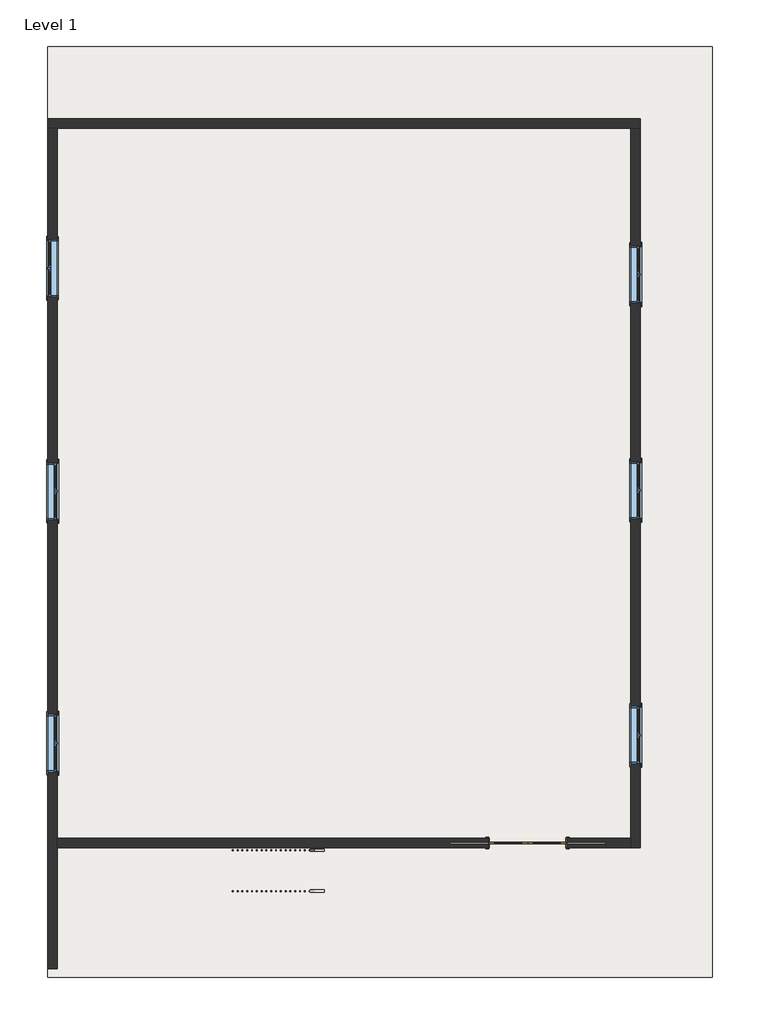
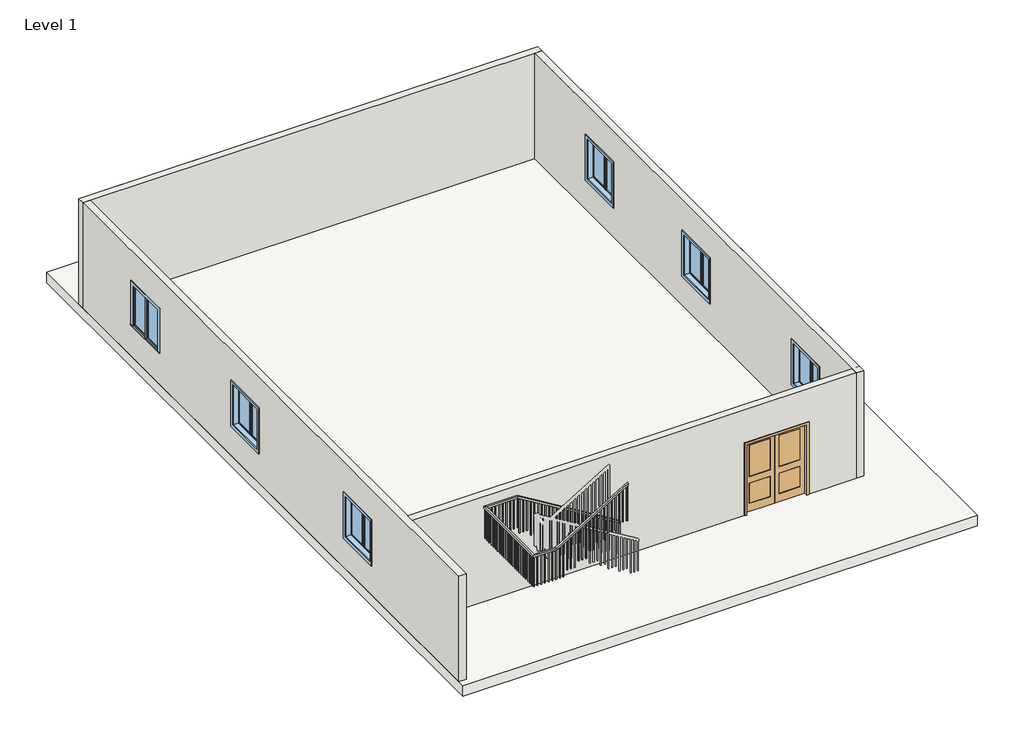
# One storey, part 1 of 2: 12 windows, 8 walls, 2 doors, 1 railing, 1 slab.
"""IFC4 building model written with IfcOpenShell, lengths in millimetres."""

from ifc_helpers import new_model, si_unit, frame, origin, origin_with_axes, place, context, project, spatial, polyline, outline, extrude, faceted_brep, transform, mapped, element, save
from components import door_18a53484, window_0862ab64

model = new_model("IFC4")

# Units and contexts
model_context = context("Model", 3, world=origin())
ifc_project = project(units=[si_unit("LENGTHUNIT", "METRE", prefix="MILLI")], contexts=[model_context])

# Site, building, storey
site = spatial("IfcSite", under=ifc_project)
building = spatial("IfcBuilding", under=site)
storey = spatial("IfcBuildingStorey", under=building, Name="Level 1", Elevation=0.0)

# Doors
placement = place(None, origin())
door_shape = door_18a53484(model_context)
element("IfcDoor", 1, ObjectType="Door-Interior-Double-Pocket-2_Panel-Wood : 64\" x 80\"", at=placement, inside=storey, context=model_context, shape_type="MappedRepresentation", body=[
    mapped(door_shape, transform((-1633.6127533, -5879.8242744, 0.0), x_axis=(1.0, 0.0, 0.0), y_axis=(0.0, 1.0, 0.0), z_axis=(0.0, 0.0, 1.0))),
])
element("IfcDoor", 2, ObjectType="Door-Interior-Double-Pocket-2_Panel-Wood : 64\" x 80\"", at=placement, inside=storey, context=model_context, shape_type="MappedRepresentation", body=[
    mapped(door_shape, transform((-1633.6127533, -5879.8242744, 0.0), x_axis=(1.0, 0.0, 0.0), y_axis=(0.0, 1.0, 0.0), z_axis=(0.0, 0.0, 1.0))),
])

# Railing
element("IfcRailing", 3, ObjectType="Handrail - Rectangular", at=placement, inside=storey, context=model_context, shape_type="SolidModel", body=[
    faceted_brep([(-5944.3382419, -6057.6242744, 1083.7333333), (-5944.3382419, -6057.6242744, 1024.3318731), (-5944.3382419, -6006.8242744, 1024.3318731), (-5944.3382419, -6006.8242744, 1083.7333333), (-8738.3382419, -6057.6242744, 2777.0666667), (-8752.5306513, -6057.6242744, 2726.2666667), (-8752.5306513, -6006.8242744, 2726.2666667), (-8738.3382419, -6006.8242744, 2777.0666667), (-9601.9382419, -6057.6242744, 2777.0666667), (-9601.9382419, -6057.6242744, 2726.2666667), (-9652.7382419, -6006.8242744, 2726.2666667), (-9652.7382419, -6006.8242744, 2777.0666667), (-9601.9382419, -8306.1243151, 2777.0666667), (-9601.9382419, -8306.1243151, 2726.2666667), (-9652.7382419, -8356.9243151, 2726.2666667), (-9652.7382419, -8356.9243151, 2777.0666667), (-9017.7382419, -8306.1243151, 2777.0666667), (-9003.5458325, -8306.1243151, 2726.2666667), (-9003.5458325, -8356.9243151, 2726.2666667), (-9017.7382419, -8356.9243151, 2777.0666667), (-7061.9382419, -8306.1243151, 3962.4), (-7061.9382419, -8356.9243151, 3962.4), (-7061.9382419, -8356.9243151, 3902.9985397), (-7061.9382419, -8306.1243151, 3902.9985397)], [[[0, 1, 2, 3]], [[1, 0, 4, 5]], [[2, 1, 5, 6]], [[3, 2, 6, 7]], [[0, 3, 7, 4]], [[5, 4, 8, 9]], [[6, 5, 9, 10]], [[7, 6, 10, 11]], [[4, 7, 11, 8]], [[9, 8, 12, 13]], [[10, 9, 13, 14]], [[11, 10, 14, 15]], [[8, 11, 15, 12]], [[13, 12, 16, 17]], [[14, 13, 17, 18]], [[15, 14, 18, 19]], [[12, 15, 19, 16]], [[20, 21, 22, 23]], [[17, 16, 20, 23]], [[18, 17, 23, 22]], [[19, 18, 22, 21]], [[16, 19, 21, 20]]]),
    extrude(outline(polyline([(3893.3773276, -7077.8132419), (3881.8318731, -7096.8632419), (2878.6666667, -7096.8632419), (2878.6666667, -7077.8132419), (3893.3773276, -7077.8132419)])), frame((0.0, -8341.0493151, 0.0), z_axis=(0.0, 1.0, 0.0), x_axis=(0.0, 0.0, 1.0)), (0.0, 0.0, 1.0), 19.05),
    extrude(outline(polyline([(3831.80157, -7179.4132419), (3820.2561155, -7198.4632419), (2878.6666667, -7198.4632419), (2878.6666667, -7179.4132419), (3831.80157, -7179.4132419)])), frame((0.0, -8341.0493151, 0.0), z_axis=(0.0, 1.0, 0.0), x_axis=(0.0, 0.0, 1.0)), (0.0, 0.0, 1.0), 19.05),
    extrude(outline(polyline([(3770.2258125, -7281.0132419), (3758.6803579, -7300.0632419), (2878.6666667, -7300.0632419), (2878.6666667, -7281.0132419), (3770.2258125, -7281.0132419)])), frame((0.0, -8341.0493151, 0.0), z_axis=(0.0, 1.0, 0.0), x_axis=(0.0, 0.0, 1.0)), (0.0, 0.0, 1.0), 19.05),
    extrude(outline(polyline([(3708.6500549, -7382.6132419), (3697.1046004, -7401.6632419), (2709.3333333, -7401.6632419), (2709.3333333, -7382.6132419), (3708.6500549, -7382.6132419)])), frame((0.0, -8341.0493151, 0.0), z_axis=(0.0, 1.0, 0.0), x_axis=(0.0, 0.0, 1.0)), (0.0, 0.0, 1.0), 19.05),
    extrude(outline(polyline([(3647.0742973, -7484.2132419), (3635.5288428, -7503.2632419), (2709.3333333, -7503.2632419), (2709.3333333, -7484.2132419), (3647.0742973, -7484.2132419)])), frame((0.0, -8341.0493151, 0.0), z_axis=(0.0, 1.0, 0.0), x_axis=(0.0, 0.0, 1.0)), (0.0, 0.0, 1.0), 19.05),
    extrude(outline(polyline([(3585.4985397, -7585.8132419), (3573.9530852, -7604.8632419), (2709.3333333, -7604.8632419), (2709.3333333, -7585.8132419), (3585.4985397, -7585.8132419)])), frame((0.0, -8341.0493151, 0.0), z_axis=(0.0, 1.0, 0.0), x_axis=(0.0, 0.0, 1.0)), (0.0, 0.0, 1.0), 19.05),
    extrude(outline(polyline([(3523.9227822, -7687.4132419), (3512.3773276, -7706.4632419), (2540.0, -7706.4632419), (2540.0, -7687.4132419), (3523.9227822, -7687.4132419)])), frame((0.0, -8341.0493151, 0.0), z_axis=(0.0, 1.0, 0.0), x_axis=(0.0, 0.0, 1.0)), (0.0, 0.0, 1.0), 19.05),
    extrude(outline(polyline([(3462.3470246, -7789.0132419), (3450.80157, -7808.0632419), (2540.0, -7808.0632419), (2540.0, -7789.0132419), (3462.3470246, -7789.0132419)])), frame((0.0, -8341.0493151, 0.0), z_axis=(0.0, 1.0, 0.0), x_axis=(0.0, 0.0, 1.0)), (0.0, 0.0, 1.0), 19.05),
    extrude(outline(polyline([(3400.771267, -7890.6132419), (3389.2258125, -7909.6632419), (2540.0, -7909.6632419), (2540.0, -7890.6132419), (3400.771267, -7890.6132419)])), frame((0.0, -8341.0493151, 0.0), z_axis=(0.0, 1.0, 0.0), x_axis=(0.0, 0.0, 1.0)), (0.0, 0.0, 1.0), 19.05),
    extrude(outline(polyline([(3339.1955094, -7992.2132419), (3327.6500549, -8011.2632419), (2370.6666667, -8011.2632419), (2370.6666667, -7992.2132419), (3339.1955094, -7992.2132419)])), frame((0.0, -8341.0493151, 0.0), z_axis=(0.0, 1.0, 0.0), x_axis=(0.0, 0.0, 1.0)), (0.0, 0.0, 1.0), 19.05),
    extrude(outline(polyline([(3277.6197519, -8093.8132419), (3266.0742973, -8112.8632419), (2370.6666667, -8112.8632419), (2370.6666667, -8093.8132419), (3277.6197519, -8093.8132419)])), frame((0.0, -8341.0493151, 0.0), z_axis=(0.0, 1.0, 0.0), x_axis=(0.0, 0.0, 1.0)), (0.0, 0.0, 1.0), 19.05),
    extrude(outline(polyline([(3216.0439943, -8195.4132419), (3204.4985397, -8214.4632419), (2201.3333333, -8214.4632419), (2201.3333333, -8195.4132419), (3216.0439943, -8195.4132419)])), frame((0.0, -8341.0493151, 0.0), z_axis=(0.0, 1.0, 0.0), x_axis=(0.0, 0.0, 1.0)), (0.0, 0.0, 1.0), 19.05),
    extrude(outline(polyline([(3154.4682367, -8297.0132419), (3142.9227822, -8316.0632419), (2201.3333333, -8316.0632419), (2201.3333333, -8297.0132419), (3154.4682367, -8297.0132419)])), frame((0.0, -8341.0493151, 0.0), z_axis=(0.0, 1.0, 0.0), x_axis=(0.0, 0.0, 1.0)), (0.0, 0.0, 1.0), 19.05),
    extrude(outline(polyline([(3092.8924791, -8398.6132419), (3081.3470246, -8417.6632419), (2201.3333333, -8417.6632419), (2201.3333333, -8398.6132419), (3092.8924791, -8398.6132419)])), frame((0.0, -8341.0493151, 0.0), z_axis=(0.0, 1.0, 0.0), x_axis=(0.0, 0.0, 1.0)), (0.0, 0.0, 1.0), 19.05),
    extrude(outline(polyline([(3031.3167216, -8500.2132419), (3019.771267, -8519.2632419), (2032.0, -8519.2632419), (2032.0, -8500.2132419), (3031.3167216, -8500.2132419)])), frame((0.0, -8341.0493151, 0.0), z_axis=(0.0, 1.0, 0.0), x_axis=(0.0, 0.0, 1.0)), (0.0, 0.0, 1.0), 19.05),
    extrude(outline(polyline([(2969.740964, -8601.8132419), (2958.1955094, -8620.8632419), (2032.0, -8620.8632419), (2032.0, -8601.8132419), (2969.740964, -8601.8132419)])), frame((0.0, -8341.0493151, 0.0), z_axis=(0.0, 1.0, 0.0), x_axis=(0.0, 0.0, 1.0)), (0.0, 0.0, 1.0), 19.05),
    extrude(outline(polyline([(2908.1652064, -8703.4132419), (2896.6197519, -8722.4632419), (2032.0, -8722.4632419), (2032.0, -8703.4132419), (2908.1652064, -8703.4132419)])), frame((0.0, -8341.0493151, 0.0), z_axis=(0.0, 1.0, 0.0), x_axis=(0.0, 0.0, 1.0)), (0.0, 0.0, 1.0), 19.05),
    extrude(outline(polyline([(2846.5894488, -8805.0132419), (2835.0439943, -8824.0632419), (1862.6666667, -8824.0632419), (1862.6666667, -8805.0132419), (2846.5894488, -8805.0132419)])), frame((0.0, -8341.0493151, 0.0), z_axis=(0.0, 1.0, 0.0), x_axis=(0.0, 0.0, 1.0)), (0.0, 0.0, 1.0), 19.05),
    extrude(outline(polyline([(2785.0136913, -8906.6132419), (2773.4682367, -8925.6632419), (1862.6666667, -8925.6632419), (1862.6666667, -8906.6132419), (2785.0136913, -8906.6132419)])), frame((0.0, -8341.0493151, 0.0), z_axis=(0.0, 1.0, 0.0), x_axis=(0.0, 0.0, 1.0)), (0.0, 0.0, 1.0), 19.05),
    extrude(outline(polyline([(-9128.8632419, -8341.0493151), (-9128.8632419, -8321.9993151), (-9109.8132419, -8321.9993151), (-9109.8132419, -8341.0493151), (-9128.8632419, -8341.0493151)])), frame((0.0, 0.0, 1862.6666667), z_axis=(0.0, 0.0, 1.0), x_axis=(1.0, 0.0, 0.0)), (0.0, 0.0, 1.0), 863.6),
    extrude(outline(polyline([(-9230.4632419, -8341.0493151), (-9230.4632419, -8321.9993151), (-9211.4132419, -8321.9993151), (-9211.4132419, -8341.0493151), (-9230.4632419, -8341.0493151)])), frame((0.0, 0.0, 1862.6666667), z_axis=(0.0, 0.0, 1.0), x_axis=(1.0, 0.0, 0.0)), (0.0, 0.0, 1.0), 863.6),
    extrude(outline(polyline([(-9332.0632419, -8341.0493151), (-9332.0632419, -8321.9993151), (-9313.0132419, -8321.9993151), (-9313.0132419, -8341.0493151), (-9332.0632419, -8341.0493151)])), frame((0.0, 0.0, 1862.6666667), z_axis=(0.0, 0.0, 1.0), x_axis=(1.0, 0.0, 0.0)), (0.0, 0.0, 1.0), 863.6),
    extrude(outline(polyline([(-9433.6632419, -8341.0493151), (-9433.6632419, -8321.9993151), (-9414.6132419, -8321.9993151), (-9414.6132419, -8341.0493151), (-9433.6632419, -8341.0493151)])), frame((0.0, 0.0, 1862.6666667), z_axis=(0.0, 0.0, 1.0), x_axis=(1.0, 0.0, 0.0)), (0.0, 0.0, 1.0), 863.6),
    extrude(outline(polyline([(-9535.2632419, -8341.0493151), (-9535.2632419, -8321.9993151), (-9516.2132419, -8321.9993151), (-9516.2132419, -8341.0493151), (-9535.2632419, -8341.0493151)])), frame((0.0, 0.0, 1862.6666667), z_axis=(0.0, 0.0, 1.0), x_axis=(1.0, 0.0, 0.0)), (0.0, 0.0, 1.0), 863.6),
    extrude(outline(polyline([(-9636.8632419, -8257.8992744), (-9617.8132419, -8257.8992744), (-9617.8132419, -8276.9492744), (-9636.8632419, -8276.9492744), (-9636.8632419, -8257.8992744)])), frame((0.0, 0.0, 1862.6666667), z_axis=(0.0, 0.0, 1.0), x_axis=(1.0, 0.0, 0.0)), (0.0, 0.0, 1.0), 863.6),
    extrude(outline(polyline([(-9636.8632419, -8156.2992744), (-9617.8132419, -8156.2992744), (-9617.8132419, -8175.3492744), (-9636.8632419, -8175.3492744), (-9636.8632419, -8156.2992744)])), frame((0.0, 0.0, 1862.6666667), z_axis=(0.0, 0.0, 1.0), x_axis=(1.0, 0.0, 0.0)), (0.0, 0.0, 1.0), 863.6),
    extrude(outline(polyline([(-9636.8632419, -8054.6992744), (-9617.8132419, -8054.6992744), (-9617.8132419, -8073.7492744), (-9636.8632419, -8073.7492744), (-9636.8632419, -8054.6992744)])), frame((0.0, 0.0, 1862.6666667), z_axis=(0.0, 0.0, 1.0), x_axis=(1.0, 0.0, 0.0)), (0.0, 0.0, 1.0), 863.6),
    extrude(outline(polyline([(-9636.8632419, -7953.0992744), (-9617.8132419, -7953.0992744), (-9617.8132419, -7972.1492744), (-9636.8632419, -7972.1492744), (-9636.8632419, -7953.0992744)])), frame((0.0, 0.0, 1862.6666667), z_axis=(0.0, 0.0, 1.0), x_axis=(1.0, 0.0, 0.0)), (0.0, 0.0, 1.0), 863.6),
    extrude(outline(polyline([(-9636.8632419, -7851.4992744), (-9617.8132419, -7851.4992744), (-9617.8132419, -7870.5492744), (-9636.8632419, -7870.5492744), (-9636.8632419, -7851.4992744)])), frame((0.0, 0.0, 1862.6666667), z_axis=(0.0, 0.0, 1.0), x_axis=(1.0, 0.0, 0.0)), (0.0, 0.0, 1.0), 863.6),
    extrude(outline(polyline([(-9636.8632419, -7749.8992744), (-9617.8132419, -7749.8992744), (-9617.8132419, -7768.9492744), (-9636.8632419, -7768.9492744), (-9636.8632419, -7749.8992744)])), frame((0.0, 0.0, 1862.6666667), z_axis=(0.0, 0.0, 1.0), x_axis=(1.0, 0.0, 0.0)), (0.0, 0.0, 1.0), 863.6),
    extrude(outline(polyline([(-9636.8632419, -7648.2992744), (-9617.8132419, -7648.2992744), (-9617.8132419, -7667.3492744), (-9636.8632419, -7667.3492744), (-9636.8632419, -7648.2992744)])), frame((0.0, 0.0, 1862.6666667), z_axis=(0.0, 0.0, 1.0), x_axis=(1.0, 0.0, 0.0)), (0.0, 0.0, 1.0), 863.6),
    extrude(outline(polyline([(-9636.8632419, -7546.6992744), (-9617.8132419, -7546.6992744), (-9617.8132419, -7565.7492744), (-9636.8632419, -7565.7492744), (-9636.8632419, -7546.6992744)])), frame((0.0, 0.0, 1862.6666667), z_axis=(0.0, 0.0, 1.0), x_axis=(1.0, 0.0, 0.0)), (0.0, 0.0, 1.0), 863.6),
    extrude(outline(polyline([(-9636.8632419, -7445.0992744), (-9617.8132419, -7445.0992744), (-9617.8132419, -7464.1492744), (-9636.8632419, -7464.1492744), (-9636.8632419, -7445.0992744)])), frame((0.0, 0.0, 1862.6666667), z_axis=(0.0, 0.0, 1.0), x_axis=(1.0, 0.0, 0.0)), (0.0, 0.0, 1.0), 863.6),
    extrude(outline(polyline([(-9636.8632419, -7343.4992744), (-9617.8132419, -7343.4992744), (-9617.8132419, -7362.5492744), (-9636.8632419, -7362.5492744), (-9636.8632419, -7343.4992744)])), frame((0.0, 0.0, 1862.6666667), z_axis=(0.0, 0.0, 1.0), x_axis=(1.0, 0.0, 0.0)), (0.0, 0.0, 1.0), 863.6),
    extrude(outline(polyline([(-9636.8632419, -7241.8992744), (-9617.8132419, -7241.8992744), (-9617.8132419, -7260.9492744), (-9636.8632419, -7260.9492744), (-9636.8632419, -7241.8992744)])), frame((0.0, 0.0, 1862.6666667), z_axis=(0.0, 0.0, 1.0), x_axis=(1.0, 0.0, 0.0)), (0.0, 0.0, 1.0), 863.6),
    extrude(outline(polyline([(-9636.8632419, -7140.2992744), (-9617.8132419, -7140.2992744), (-9617.8132419, -7159.3492744), (-9636.8632419, -7159.3492744), (-9636.8632419, -7140.2992744)])), frame((0.0, 0.0, 1862.6666667), z_axis=(0.0, 0.0, 1.0), x_axis=(1.0, 0.0, 0.0)), (0.0, 0.0, 1.0), 863.6),
    extrude(outline(polyline([(-9636.8632419, -7038.6992744), (-9617.8132419, -7038.6992744), (-9617.8132419, -7057.7492744), (-9636.8632419, -7057.7492744), (-9636.8632419, -7038.6992744)])), frame((0.0, 0.0, 1862.6666667), z_axis=(0.0, 0.0, 1.0), x_axis=(1.0, 0.0, 0.0)), (0.0, 0.0, 1.0), 863.6),
    extrude(outline(polyline([(-9636.8632419, -6937.0992744), (-9617.8132419, -6937.0992744), (-9617.8132419, -6956.1492744), (-9636.8632419, -6956.1492744), (-9636.8632419, -6937.0992744)])), frame((0.0, 0.0, 1862.6666667), z_axis=(0.0, 0.0, 1.0), x_axis=(1.0, 0.0, 0.0)), (0.0, 0.0, 1.0), 863.6),
    extrude(outline(polyline([(-9636.8632419, -6835.4992744), (-9617.8132419, -6835.4992744), (-9617.8132419, -6854.5492744), (-9636.8632419, -6854.5492744), (-9636.8632419, -6835.4992744)])), frame((0.0, 0.0, 1862.6666667), z_axis=(0.0, 0.0, 1.0), x_axis=(1.0, 0.0, 0.0)), (0.0, 0.0, 1.0), 863.6),
    extrude(outline(polyline([(-9636.8632419, -6733.8992744), (-9617.8132419, -6733.8992744), (-9617.8132419, -6752.9492744), (-9636.8632419, -6752.9492744), (-9636.8632419, -6733.8992744)])), frame((0.0, 0.0, 1862.6666667), z_axis=(0.0, 0.0, 1.0), x_axis=(1.0, 0.0, 0.0)), (0.0, 0.0, 1.0), 863.6),
    extrude(outline(polyline([(-9636.8632419, -6632.2992744), (-9617.8132419, -6632.2992744), (-9617.8132419, -6651.3492744), (-9636.8632419, -6651.3492744), (-9636.8632419, -6632.2992744)])), frame((0.0, 0.0, 1862.6666667), z_axis=(0.0, 0.0, 1.0), x_axis=(1.0, 0.0, 0.0)), (0.0, 0.0, 1.0), 863.6),
    extrude(outline(polyline([(-9636.8632419, -6530.6992744), (-9617.8132419, -6530.6992744), (-9617.8132419, -6549.7492744), (-9636.8632419, -6549.7492744), (-9636.8632419, -6530.6992744)])), frame((0.0, 0.0, 1862.6666667), z_axis=(0.0, 0.0, 1.0), x_axis=(1.0, 0.0, 0.0)), (0.0, 0.0, 1.0), 863.6),
    extrude(outline(polyline([(-9636.8632419, -6429.0992744), (-9617.8132419, -6429.0992744), (-9617.8132419, -6448.1492744), (-9636.8632419, -6448.1492744), (-9636.8632419, -6429.0992744)])), frame((0.0, 0.0, 1862.6666667), z_axis=(0.0, 0.0, 1.0), x_axis=(1.0, 0.0, 0.0)), (0.0, 0.0, 1.0), 863.6),
    extrude(outline(polyline([(-9636.8632419, -6327.4992744), (-9617.8132419, -6327.4992744), (-9617.8132419, -6346.5492744), (-9636.8632419, -6346.5492744), (-9636.8632419, -6327.4992744)])), frame((0.0, 0.0, 1862.6666667), z_axis=(0.0, 0.0, 1.0), x_axis=(1.0, 0.0, 0.0)), (0.0, 0.0, 1.0), 863.6),
    extrude(outline(polyline([(-9636.8632419, -6225.8992744), (-9617.8132419, -6225.8992744), (-9617.8132419, -6244.9492744), (-9636.8632419, -6244.9492744), (-9636.8632419, -6225.8992744)])), frame((0.0, 0.0, 1862.6666667), z_axis=(0.0, 0.0, 1.0), x_axis=(1.0, 0.0, 0.0)), (0.0, 0.0, 1.0), 863.6),
    extrude(outline(polyline([(-9636.8632419, -6124.2992744), (-9617.8132419, -6124.2992744), (-9617.8132419, -6143.3492744), (-9636.8632419, -6143.3492744), (-9636.8632419, -6124.2992744)])), frame((0.0, 0.0, 1862.6666667), z_axis=(0.0, 0.0, 1.0), x_axis=(1.0, 0.0, 0.0)), (0.0, 0.0, 1.0), 863.6),
    extrude(outline(polyline([(-9541.6132419, -6022.6992744), (-9541.6132419, -6041.7492744), (-9560.6632419, -6041.7492744), (-9560.6632419, -6022.6992744), (-9541.6132419, -6022.6992744)])), frame((0.0, 0.0, 1862.6666667), z_axis=(0.0, 0.0, 1.0), x_axis=(1.0, 0.0, 0.0)), (0.0, 0.0, 1.0), 863.6),
    extrude(outline(polyline([(-9440.0132419, -6022.6992744), (-9440.0132419, -6041.7492744), (-9459.0632419, -6041.7492744), (-9459.0632419, -6022.6992744), (-9440.0132419, -6022.6992744)])), frame((0.0, 0.0, 1862.6666667), z_axis=(0.0, 0.0, 1.0), x_axis=(1.0, 0.0, 0.0)), (0.0, 0.0, 1.0), 863.6),
    extrude(outline(polyline([(-9338.4132419, -6022.6992744), (-9338.4132419, -6041.7492744), (-9357.4632419, -6041.7492744), (-9357.4632419, -6022.6992744), (-9338.4132419, -6022.6992744)])), frame((0.0, 0.0, 1862.6666667), z_axis=(0.0, 0.0, 1.0), x_axis=(1.0, 0.0, 0.0)), (0.0, 0.0, 1.0), 863.6),
    extrude(outline(polyline([(-9236.8132419, -6022.6992744), (-9236.8132419, -6041.7492744), (-9255.8632419, -6041.7492744), (-9255.8632419, -6022.6992744), (-9236.8132419, -6022.6992744)])), frame((0.0, 0.0, 1862.6666667), z_axis=(0.0, 0.0, 1.0), x_axis=(1.0, 0.0, 0.0)), (0.0, 0.0, 1.0), 863.6),
    extrude(outline(polyline([(-9135.2132419, -6022.6992744), (-9135.2132419, -6041.7492744), (-9154.2632419, -6041.7492744), (-9154.2632419, -6022.6992744), (-9135.2132419, -6022.6992744)])), frame((0.0, 0.0, 1862.6666667), z_axis=(0.0, 0.0, 1.0), x_axis=(1.0, 0.0, 0.0)), (0.0, 0.0, 1.0), 863.6),
    extrude(outline(polyline([(-9033.6132419, -6022.6992744), (-9033.6132419, -6041.7492744), (-9052.6632419, -6041.7492744), (-9052.6632419, -6022.6992744), (-9033.6132419, -6022.6992744)])), frame((0.0, 0.0, 1862.6666667), z_axis=(0.0, 0.0, 1.0), x_axis=(1.0, 0.0, 0.0)), (0.0, 0.0, 1.0), 863.6),
    extrude(outline(polyline([(-8932.0132419, -6022.6992744), (-8932.0132419, -6041.7492744), (-8951.0632419, -6041.7492744), (-8951.0632419, -6022.6992744), (-8932.0132419, -6022.6992744)])), frame((0.0, 0.0, 1862.6666667), z_axis=(0.0, 0.0, 1.0), x_axis=(1.0, 0.0, 0.0)), (0.0, 0.0, 1.0), 863.6),
    extrude(outline(polyline([(-8830.4132419, -6022.6992744), (-8830.4132419, -6041.7492744), (-8849.4632419, -6041.7492744), (-8849.4632419, -6022.6992744), (-8830.4132419, -6022.6992744)])), frame((0.0, 0.0, 1862.6666667), z_axis=(0.0, 0.0, 1.0), x_axis=(1.0, 0.0, 0.0)), (0.0, 0.0, 1.0), 863.6),
    extrude(outline(polyline([(2681.1046004, -8678.0132419), (2692.6500549, -8697.0632419), (1693.3333333, -8697.0632419), (1693.3333333, -8678.0132419), (2681.1046004, -8678.0132419)])), frame((0.0, -6041.7492744, 0.0), z_axis=(0.0, 1.0, 0.0), x_axis=(0.0, 0.0, 1.0)), (0.0, 0.0, 1.0), 19.05),
    extrude(outline(polyline([(2619.5288428, -8576.4132419), (2631.0742973, -8595.4632419), (1693.3333333, -8595.4632419), (1693.3333333, -8576.4132419), (2619.5288428, -8576.4132419)])), frame((0.0, -6041.7492744, 0.0), z_axis=(0.0, 1.0, 0.0), x_axis=(0.0, 0.0, 1.0)), (0.0, 0.0, 1.0), 19.05),
    extrude(outline(polyline([(2557.9530852, -8474.8132419), (2569.4985397, -8493.8632419), (1693.3333333, -8493.8632419), (1693.3333333, -8474.8132419), (2557.9530852, -8474.8132419)])), frame((0.0, -6041.7492744, 0.0), z_axis=(0.0, 1.0, 0.0), x_axis=(0.0, 0.0, 1.0)), (0.0, 0.0, 1.0), 19.05),
    extrude(outline(polyline([(2496.3773276, -8373.2132419), (2507.9227822, -8392.2632419), (1524.0, -8392.2632419), (1524.0, -8373.2132419), (2496.3773276, -8373.2132419)])), frame((0.0, -6041.7492744, 0.0), z_axis=(0.0, 1.0, 0.0), x_axis=(0.0, 0.0, 1.0)), (0.0, 0.0, 1.0), 19.05),
    extrude(outline(polyline([(2434.80157, -8271.6132419), (2446.3470246, -8290.6632419), (1524.0, -8290.6632419), (1524.0, -8271.6132419), (2434.80157, -8271.6132419)])), frame((0.0, -6041.7492744, 0.0), z_axis=(0.0, 1.0, 0.0), x_axis=(0.0, 0.0, 1.0)), (0.0, 0.0, 1.0), 19.05),
    extrude(outline(polyline([(2373.2258125, -8170.0132419), (2384.771267, -8189.0632419), (1524.0, -8189.0632419), (1524.0, -8170.0132419), (2373.2258125, -8170.0132419)])), frame((0.0, -6041.7492744, 0.0), z_axis=(0.0, 1.0, 0.0), x_axis=(0.0, 0.0, 1.0)), (0.0, 0.0, 1.0), 19.05),
    extrude(outline(polyline([(2311.6500549, -8068.4132419), (2323.1955094, -8087.4632419), (1354.6666667, -8087.4632419), (1354.6666667, -8068.4132419), (2311.6500549, -8068.4132419)])), frame((0.0, -6041.7492744, 0.0), z_axis=(0.0, 1.0, 0.0), x_axis=(0.0, 0.0, 1.0)), (0.0, 0.0, 1.0), 19.05),
    extrude(outline(polyline([(2250.0742973, -7966.8132419), (2261.6197519, -7985.8632419), (1354.6666667, -7985.8632419), (1354.6666667, -7966.8132419), (2250.0742973, -7966.8132419)])), frame((0.0, -6041.7492744, 0.0), z_axis=(0.0, 1.0, 0.0), x_axis=(0.0, 0.0, 1.0)), (0.0, 0.0, 1.0), 19.05),
    extrude(outline(polyline([(2188.4985397, -7865.2132419), (2200.0439943, -7884.2632419), (1185.3333333, -7884.2632419), (1185.3333333, -7865.2132419), (2188.4985397, -7865.2132419)])), frame((0.0, -6041.7492744, 0.0), z_axis=(0.0, 1.0, 0.0), x_axis=(0.0, 0.0, 1.0)), (0.0, 0.0, 1.0), 19.05),
    extrude(outline(polyline([(2126.9227822, -7763.6132419), (2138.4682367, -7782.6632419), (1185.3333333, -7782.6632419), (1185.3333333, -7763.6132419), (2126.9227822, -7763.6132419)])), frame((0.0, -6041.7492744, 0.0), z_axis=(0.0, 1.0, 0.0), x_axis=(0.0, 0.0, 1.0)), (0.0, 0.0, 1.0), 19.05),
    extrude(outline(polyline([(2065.3470246, -7662.0132419), (2076.8924791, -7681.0632419), (1185.3333333, -7681.0632419), (1185.3333333, -7662.0132419), (2065.3470246, -7662.0132419)])), frame((0.0, -6041.7492744, 0.0), z_axis=(0.0, 1.0, 0.0), x_axis=(0.0, 0.0, 1.0)), (0.0, 0.0, 1.0), 19.05),
    extrude(outline(polyline([(2003.771267, -7560.4132419), (2015.3167216, -7579.4632419), (1016.0, -7579.4632419), (1016.0, -7560.4132419), (2003.771267, -7560.4132419)])), frame((0.0, -6041.7492744, 0.0), z_axis=(0.0, 1.0, 0.0), x_axis=(0.0, 0.0, 1.0)), (0.0, 0.0, 1.0), 19.05),
    extrude(outline(polyline([(1942.1955094, -7458.8132419), (1953.740964, -7477.8632419), (1016.0, -7477.8632419), (1016.0, -7458.8132419), (1942.1955094, -7458.8132419)])), frame((0.0, -6041.7492744, 0.0), z_axis=(0.0, 1.0, 0.0), x_axis=(0.0, 0.0, 1.0)), (0.0, 0.0, 1.0), 19.05),
    extrude(outline(polyline([(1880.6197519, -7357.2132419), (1892.1652064, -7376.2632419), (1016.0, -7376.2632419), (1016.0, -7357.2132419), (1880.6197519, -7357.2132419)])), frame((0.0, -6041.7492744, 0.0), z_axis=(0.0, 1.0, 0.0), x_axis=(0.0, 0.0, 1.0)), (0.0, 0.0, 1.0), 19.05),
    extrude(outline(polyline([(1819.0439943, -7255.6132419), (1830.5894488, -7274.6632419), (846.6666667, -7274.6632419), (846.6666667, -7255.6132419), (1819.0439943, -7255.6132419)])), frame((0.0, -6041.7492744, 0.0), z_axis=(0.0, 1.0, 0.0), x_axis=(0.0, 0.0, 1.0)), (0.0, 0.0, 1.0), 19.05),
    extrude(outline(polyline([(1757.4682367, -7154.0132419), (1769.0136913, -7173.0632419), (846.6666667, -7173.0632419), (846.6666667, -7154.0132419), (1757.4682367, -7154.0132419)])), frame((0.0, -6041.7492744, 0.0), z_axis=(0.0, 1.0, 0.0), x_axis=(0.0, 0.0, 1.0)), (0.0, 0.0, 1.0), 19.05),
    extrude(outline(polyline([(1695.8924791, -7052.4132419), (1707.4379337, -7071.4632419), (846.6666667, -7071.4632419), (846.6666667, -7052.4132419), (1695.8924791, -7052.4132419)])), frame((0.0, -6041.7492744, 0.0), z_axis=(0.0, 1.0, 0.0), x_axis=(0.0, 0.0, 1.0)), (0.0, 0.0, 1.0), 19.05),
    extrude(outline(polyline([(1634.3167216, -6950.8132419), (1645.8621761, -6969.8632419), (677.3333333, -6969.8632419), (677.3333333, -6950.8132419), (1634.3167216, -6950.8132419)])), frame((0.0, -6041.7492744, 0.0), z_axis=(0.0, 1.0, 0.0), x_axis=(0.0, 0.0, 1.0)), (0.0, 0.0, 1.0), 19.05),
    extrude(outline(polyline([(1572.740964, -6849.2132419), (1584.2864185, -6868.2632419), (677.3333333, -6868.2632419), (677.3333333, -6849.2132419), (1572.740964, -6849.2132419)])), frame((0.0, -6041.7492744, 0.0), z_axis=(0.0, 1.0, 0.0), x_axis=(0.0, 0.0, 1.0)), (0.0, 0.0, 1.0), 19.05),
    extrude(outline(polyline([(1511.1652064, -6747.6132419), (1522.710661, -6766.6632419), (508.0, -6766.6632419), (508.0, -6747.6132419), (1511.1652064, -6747.6132419)])), frame((0.0, -6041.7492744, 0.0), z_axis=(0.0, 1.0, 0.0), x_axis=(0.0, 0.0, 1.0)), (0.0, 0.0, 1.0), 19.05),
    extrude(outline(polyline([(1449.5894488, -6646.0132419), (1461.1349034, -6665.0632419), (508.0, -6665.0632419), (508.0, -6646.0132419), (1449.5894488, -6646.0132419)])), frame((0.0, -6041.7492744, 0.0), z_axis=(0.0, 1.0, 0.0), x_axis=(0.0, 0.0, 1.0)), (0.0, 0.0, 1.0), 19.05),
    extrude(outline(polyline([(1388.0136913, -6544.4132419), (1399.5591458, -6563.4632419), (508.0, -6563.4632419), (508.0, -6544.4132419), (1388.0136913, -6544.4132419)])), frame((0.0, -6041.7492744, 0.0), z_axis=(0.0, 1.0, 0.0), x_axis=(0.0, 0.0, 1.0)), (0.0, 0.0, 1.0), 19.05),
    extrude(outline(polyline([(1326.4379337, -6442.8132419), (1337.9833882, -6461.8632419), (338.6666667, -6461.8632419), (338.6666667, -6442.8132419), (1326.4379337, -6442.8132419)])), frame((0.0, -6041.7492744, 0.0), z_axis=(0.0, 1.0, 0.0), x_axis=(0.0, 0.0, 1.0)), (0.0, 0.0, 1.0), 19.05),
    extrude(outline(polyline([(1264.8621761, -6341.2132419), (1276.4076307, -6360.2632419), (338.6666667, -6360.2632419), (338.6666667, -6341.2132419), (1264.8621761, -6341.2132419)])), frame((0.0, -6041.7492744, 0.0), z_axis=(0.0, 1.0, 0.0), x_axis=(0.0, 0.0, 1.0)), (0.0, 0.0, 1.0), 19.05),
    extrude(outline(polyline([(1203.2864185, -6239.6132419), (1214.8318731, -6258.6632419), (338.6666667, -6258.6632419), (338.6666667, -6239.6132419), (1203.2864185, -6239.6132419)])), frame((0.0, -6041.7492744, 0.0), z_axis=(0.0, 1.0, 0.0), x_axis=(0.0, 0.0, 1.0)), (0.0, 0.0, 1.0), 19.05),
    extrude(outline(polyline([(1141.710661, -6138.0132419), (1153.2561155, -6157.0632419), (169.3333333, -6157.0632419), (169.3333333, -6138.0132419), (1141.710661, -6138.0132419)])), frame((0.0, -6041.7492744, 0.0), z_axis=(0.0, 1.0, 0.0), x_axis=(0.0, 0.0, 1.0)), (0.0, 0.0, 1.0), 19.05),
    extrude(outline(polyline([(1080.1349034, -6036.4132419), (1091.6803579, -6055.4632419), (169.3333333, -6055.4632419), (169.3333333, -6036.4132419), (1080.1349034, -6036.4132419)])), frame((0.0, -6041.7492744, 0.0), z_axis=(0.0, 1.0, 0.0), x_axis=(0.0, 0.0, 1.0)), (0.0, 0.0, 1.0), 19.05),
    extrude(outline(polyline([(-9027.2632419, -8341.0493151), (-9027.2632419, -8321.9993151), (-9008.2132419, -8321.9993151), (-9008.2132419, -8341.0493151), (-9027.2632419, -8341.0493151)])), frame((0.0, 0.0, 1862.6666667), z_axis=(0.0, 0.0, 1.0), x_axis=(1.0, 0.0, 0.0)), (0.0, 0.0, 1.0), 863.6),
    extrude(outline(polyline([(-9636.8632419, -8321.9993151), (-9617.8132419, -8321.9993151), (-9617.8132419, -8341.0493151), (-9636.8632419, -8341.0493151), (-9636.8632419, -8321.9993151)])), frame((0.0, 0.0, 1862.6666667), z_axis=(0.0, 0.0, 1.0), x_axis=(1.0, 0.0, 0.0)), (0.0, 0.0, 1.0), 863.6),
    extrude(outline(polyline([(-9617.8132419, -6022.6992744), (-9617.8132419, -6041.7492744), (-9636.8632419, -6041.7492744), (-9636.8632419, -6022.6992744), (-9617.8132419, -6022.6992744)])), frame((0.0, 0.0, 1862.6666667), z_axis=(0.0, 0.0, 1.0), x_axis=(1.0, 0.0, 0.0)), (0.0, 0.0, 1.0), 863.6),
    extrude(outline(polyline([(2711.8924791, -8728.8132419), (2723.4379337, -8747.8632419), (1862.6666667, -8747.8632419), (1862.6666667, -8728.8132419), (2711.8924791, -8728.8132419)])), frame((0.0, -6041.7492744, 0.0), z_axis=(0.0, 1.0, 0.0), x_axis=(0.0, 0.0, 1.0)), (0.0, 0.0, 1.0), 19.05),
    extrude(outline(polyline([(3902.9985397, -7061.9382419), (3891.4530852, -7080.9882419), (2878.6666667, -7080.9882419), (2878.6666667, -7061.9382419), (3902.9985397, -7061.9382419)])), frame((0.0, -8341.0493151, 0.0), z_axis=(0.0, 1.0, 0.0), x_axis=(0.0, 0.0, 1.0)), (0.0, 0.0, 1.0), 19.05),
    extrude(outline(polyline([(1024.3318731, -5944.3382419), (1035.8773276, -5963.3882419), (169.3333333, -5963.3882419), (169.3333333, -5944.3382419), (1024.3318731, -5944.3382419)])), frame((0.0, -6041.7492744, 0.0), z_axis=(0.0, 1.0, 0.0), x_axis=(0.0, 0.0, 1.0)), (0.0, 0.0, 1.0), 19.05),
])

# Slab
element("IfcSlab", 4, ObjectType="Generic - 12\"", at=placement, inside=storey, context=model_context, shape_type="SweptSolid", body=[
    extrude(outline(polyline([(-11793.6127533, 10985.7757256), (2277.9872467, 10985.7757256), (2277.9872467, -8724.6242744), (-11793.6127533, -8724.6242744), (-11793.6127533, 10985.7757256)])), frame((0.0, 0.0, -304.8), z_axis=(0.0, 0.0, 1.0), x_axis=(1.0, 0.0, 0.0)), (0.0, 0.0, 1.0), 304.8),
])

# Walls
element("IfcWall", 5, ObjectType="Generic - 8\"", at=placement, inside=storey, context=model_context, shape_type="Brep", body=[
    faceted_brep([(-11793.6127533, 9258.5757256, 0.0), (-11590.4127533, 9258.5757256, 0.0), (550.7872467, 9258.5757256, 0.0), (753.9872467, 9258.5757256, 0.0), (753.9872467, 9258.5757256, 3048.0), (550.7872467, 9258.5757256, 3048.0), (-11590.4127533, 9258.5757256, 3048.0), (-11793.6127533, 9258.5757256, 3048.0), (-11793.6127533, 9461.7757256, 0.0), (-11793.6127533, 9461.7757256, 3048.0), (753.9872467, 9461.7757256, 3048.0), (753.9872467, 9461.7757256, 0.0)], [[[0, 1, 2, 3, 4, 5, 6, 7]], [[8, 9, 10, 11]], [[3, 2, 1, 0, 8, 11]], [[7, 6, 5, 4, 10, 9]], [[4, 3, 11, 10]], [[0, 7, 9, 8]]]),
])
element("IfcWall", 6, ObjectType="Generic - 8\"", at=placement, inside=storey, context=model_context, shape_type="Brep", body=[
    faceted_brep([(550.7872467, 9258.5757256, 0.0), (550.7872467, -5778.2242744, 0.0), (550.7872467, -5981.4242744, 0.0), (550.7872467, -5981.4242744, 3048.0), (550.7872467, -5778.2242744, 3048.0), (550.7872467, 9258.5757256, 3048.0), (550.7872467, -4203.4242744, 2133.6), (550.7872467, -4203.4242744, 914.4), (550.7872467, -2984.2242744, 914.4), (550.7872467, -2984.2242744, 2133.6), (550.7872467, 978.1757256, 2133.6), (550.7872467, 978.1757256, 914.4), (550.7872467, 2197.3757256, 914.4), (550.7872467, 2197.3757256, 2133.6), (550.7872467, 5550.1757256, 2133.6), (550.7872467, 5550.1757256, 914.4), (550.7872467, 6769.3757256, 914.4), (550.7872467, 6769.3757256, 2133.6), (753.9872467, 9258.5757256, 0.0), (753.9872467, 9258.5757256, 3048.0), (753.9872467, -5981.4242744, 3048.0), (753.9872467, -5981.4242744, 0.0), (753.9872467, -4203.4242744, 2133.6), (753.9872467, -2984.2242744, 2133.6), (753.9872467, -2984.2242744, 914.4), (753.9872467, -4203.4242744, 914.4), (753.9872467, 978.1757256, 2133.6), (753.9872467, 2197.3757256, 2133.6), (753.9872467, 2197.3757256, 914.4), (753.9872467, 978.1757256, 914.4), (753.9872467, 5550.1757256, 2133.6), (753.9872467, 6769.3757256, 2133.6), (753.9872467, 6769.3757256, 914.4), (753.9872467, 5550.1757256, 914.4)], [[[0, 1, 2, 3, 4, 5], [6, 7, 8, 9], [10, 11, 12, 13], [14, 15, 16, 17]], [[18, 19, 20, 21], [22, 23, 24, 25], [26, 27, 28, 29], [30, 31, 32, 33]], [[2, 1, 0, 18, 21]], [[5, 4, 3, 20, 19]], [[0, 5, 19, 18]], [[3, 2, 21, 20]], [[7, 6, 22, 25]], [[8, 7, 25, 24]], [[9, 8, 24, 23]], [[6, 9, 23, 22]], [[11, 10, 26, 29]], [[12, 11, 29, 28]], [[13, 12, 28, 27]], [[10, 13, 27, 26]], [[15, 14, 30, 33]], [[16, 15, 33, 32]], [[17, 16, 32, 31]], [[14, 17, 31, 30]]]),
])
element("IfcWall", 7, ObjectType="Generic - 8\"", at=placement, inside=storey, context=model_context, shape_type="Brep", body=[
    faceted_brep([(-11590.4127533, -5778.2242744, 3048.0), (550.7872467, -5778.2242744, 3048.0), (550.7872467, -5778.2242744, 0.0), (-795.4127533, -5778.2242744, 0.0), (-795.4127533, -5778.2242744, 2057.4), (-2471.8127533, -5778.2242744, 2057.4), (-2471.8127533, -5778.2242744, 0.0), (-11590.4127533, -5778.2242744, 0.0), (550.7872467, -5981.4242744, 3048.0), (-11590.4127533, -5981.4242744, 3048.0), (-11590.4127533, -5981.4242744, 0.0), (-2471.8127533, -5981.4242744, 0.0), (-2471.8127533, -5981.4242744, 2057.4), (-795.4127533, -5981.4242744, 2057.4), (-795.4127533, -5981.4242744, 0.0), (550.7872467, -5981.4242744, 0.0), (-795.4127533, -5900.4617744, 0.0), (17.3872467, -5900.4617744, 0.0), (17.3872467, -5859.1867744, 0.0), (-795.4127533, -5859.1867744, 0.0), (-2471.8127533, -5859.1867744, 0.0), (-3284.6127533, -5859.1867744, 0.0), (-3284.6127533, -5900.4617744, 0.0), (-2471.8127533, -5900.4617744, 0.0), (17.3872467, -5859.1867744, 2057.4), (17.3872467, -5900.4617744, 2057.4), (-795.4127533, -5900.4617744, 2057.4), (-2471.8127533, -5900.4617744, 2057.4), (-3284.6127533, -5900.4617744, 2057.4), (-3284.6127533, -5859.1867744, 2057.4), (-2471.8127533, -5859.1867744, 2057.4), (-795.4127533, -5859.1867744, 2057.4)], [[[0, 1, 2, 3, 4, 5, 6, 7]], [[8, 9, 10, 11, 12, 13, 14, 15]], [[2, 15, 14, 16, 17, 18, 19, 3]], [[10, 7, 6, 20, 21, 22, 23, 11]], [[1, 0, 9, 8]], [[2, 1, 8, 15]], [[0, 7, 10, 9]], [[24, 25, 26, 13, 12, 27, 28, 29, 30, 5, 4, 31]], [[24, 31, 19, 18]], [[31, 4, 3, 19]], [[5, 30, 20, 6]], [[30, 29, 21, 20]], [[29, 28, 22, 21]], [[28, 27, 23, 22]], [[27, 12, 11, 23]], [[13, 26, 16, 14]], [[26, 25, 17, 16]], [[25, 24, 18, 17]]]),
])
element("IfcWall", 8, ObjectType="Generic - 8\"", at=placement, inside=storey, context=model_context, shape_type="Brep", body=[
    faceted_brep([(-11590.4127533, -8542.0083309, 0.0), (-11590.4127533, -5981.4242744, 0.0), (-11590.4127533, -5778.2242744, 0.0), (-11590.4127533, 9258.5757256, 0.0), (-11590.4127533, 9258.5757256, 3048.0), (-11590.4127533, -5778.2242744, 3048.0), (-11590.4127533, -5981.4242744, 3048.0), (-11590.4127533, -8542.0083309, 3048.0), (-11590.4127533, 6901.1916691, 2133.6), (-11590.4127533, 6901.1916691, 914.4), (-11590.4127533, 5681.9916691, 914.4), (-11590.4127533, 5681.9916691, 2133.6), (-11590.4127533, 957.5916691, 2133.6), (-11590.4127533, 2176.7916691, 2133.6), (-11590.4127533, 2176.7916691, 914.4), (-11590.4127533, 957.5916691, 914.4), (-11590.4127533, -4376.4083309, 2133.6), (-11590.4127533, -3157.2083309, 2133.6), (-11590.4127533, -3157.2083309, 914.4), (-11590.4127533, -4376.4083309, 914.4), (-11793.6127533, -8542.0083309, 0.0), (-11793.6127533, -8542.0083309, 3048.0), (-11793.6127533, 9258.5757256, 3048.0), (-11793.6127533, 9258.5757256, 0.0), (-11793.6127533, 6901.1916691, 2133.6), (-11793.6127533, 5681.9916691, 2133.6), (-11793.6127533, 5681.9916691, 914.4), (-11793.6127533, 6901.1916691, 914.4), (-11793.6127533, 957.5916691, 2133.6), (-11793.6127533, 957.5916691, 914.4), (-11793.6127533, 2176.7916691, 914.4), (-11793.6127533, 2176.7916691, 2133.6), (-11793.6127533, -4376.4083309, 2133.6), (-11793.6127533, -4376.4083309, 914.4), (-11793.6127533, -3157.2083309, 914.4), (-11793.6127533, -3157.2083309, 2133.6)], [[[0, 1, 2, 3, 4, 5, 6, 7], [8, 9, 10, 11], [12, 13, 14, 15], [16, 17, 18, 19]], [[20, 21, 22, 23], [24, 25, 26, 27], [28, 29, 30, 31], [32, 33, 34, 35]], [[3, 2, 1, 0, 20, 23]], [[7, 6, 5, 4, 22, 21]], [[0, 7, 21, 20]], [[4, 3, 23, 22]], [[9, 8, 24, 27]], [[10, 9, 27, 26]], [[11, 10, 26, 25]], [[8, 11, 25, 24]], [[29, 28, 12, 15]], [[30, 29, 15, 14]], [[31, 30, 14, 13]], [[28, 31, 13, 12]], [[33, 32, 16, 19]], [[34, 33, 19, 18]], [[35, 34, 18, 17]], [[32, 35, 17, 16]]]),
])
element("IfcWall", 9, ObjectType="Generic - 8\"", at=placement, inside=storey, context=model_context, shape_type="SweptSolid", body=[
    extrude(outline(polyline([(550.7872467, 9258.5757256), (-11590.4127533, 9258.5757256), (-11590.4127533, 9461.7757256), (550.7872467, 9461.7757256), (550.7872467, 9258.5757256)])), origin_with_axes(), (0.0, 0.0, 1.0), 3048.0),
])
element("IfcWall", 10, ObjectType="Generic - 8\"", at=placement, inside=storey, context=model_context, shape_type="SweptSolid", body=[
    extrude(outline(polyline([(9258.5757256, 0.0), (-5778.2242744, 0.0), (-5778.2242744, 3048.0), (9258.5757256, 3048.0), (9258.5757256, 0.0)]), holes=[polyline([(-4203.4242744, 2133.6), (-4203.4242744, 914.4), (-2984.2242744, 914.4), (-2984.2242744, 2133.6), (-4203.4242744, 2133.6)]), polyline([(978.1757256, 2133.6), (978.1757256, 914.4), (2197.3757256, 914.4), (2197.3757256, 2133.6), (978.1757256, 2133.6)]), polyline([(5550.1757256, 2133.6), (5550.1757256, 914.4), (6769.3757256, 914.4), (6769.3757256, 2133.6), (5550.1757256, 2133.6)])]), frame((550.7872467, 0.0, 0.0), z_axis=(1.0, 0.0, 0.0), x_axis=(0.0, 1.0, 0.0)), (0.0, 0.0, 1.0), 203.2),
])
element("IfcWall", 11, ObjectType="Generic - 8\"", at=placement, inside=storey, context=model_context, shape_type="Brep", body=[
    faceted_brep([(-11590.4127533, -5778.2242744, 3048.0), (550.7872467, -5778.2242744, 3048.0), (550.7872467, -5778.2242744, 0.0), (-795.4127533, -5778.2242744, 0.0), (-795.4127533, -5778.2242744, 2057.4), (-2471.8127533, -5778.2242744, 2057.4), (-2471.8127533, -5778.2242744, 0.0), (-11590.4127533, -5778.2242744, 0.0), (550.7872467, -5981.4242744, 3048.0), (-11590.4127533, -5981.4242744, 3048.0), (-11590.4127533, -5981.4242744, 0.0), (-2471.8127533, -5981.4242744, 0.0), (-2471.8127533, -5981.4242744, 2057.4), (-795.4127533, -5981.4242744, 2057.4), (-795.4127533, -5981.4242744, 0.0), (550.7872467, -5981.4242744, 0.0), (-795.4127533, -5900.4617744, 0.0), (17.3872467, -5900.4617744, 0.0), (17.3872467, -5859.1867744, 0.0), (-795.4127533, -5859.1867744, 0.0), (-795.4127533, -5859.1867744, 2057.4), (17.3872467, -5859.1867744, 2057.4), (17.3872467, -5900.4617744, 2057.4), (-795.4127533, -5900.4617744, 2057.4), (-2471.8127533, -5900.4617744, 2057.4), (-3284.6127533, -5900.4617744, 2057.4), (-3284.6127533, -5859.1867744, 2057.4), (-2471.8127533, -5859.1867744, 2057.4), (-2471.8127533, -5859.1867744, 0.0), (-3284.6127533, -5859.1867744, 0.0), (-3284.6127533, -5900.4617744, 0.0), (-2471.8127533, -5900.4617744, 0.0)], [[[0, 1, 2, 3, 4, 5, 6, 7]], [[8, 9, 10, 11, 12, 13, 14, 15]], [[3, 2, 15, 14, 16, 17, 18, 19]], [[1, 0, 9, 8]], [[0, 7, 10, 9]], [[5, 4, 20, 21, 22, 23, 13, 12, 24, 25, 26, 27]], [[19, 18, 21, 20]], [[4, 3, 19, 20]], [[6, 5, 27, 28]], [[29, 28, 27, 26]], [[30, 29, 26, 25]], [[31, 30, 25, 24]], [[12, 11, 31, 24]], [[14, 13, 23, 16]], [[17, 16, 23, 22]], [[18, 17, 22, 21]], [[2, 1, 8, 15]], [[7, 6, 28, 29, 30, 31, 11, 10]]]),
])
element("IfcWall", 12, ObjectType="Generic - 8\"", at=placement, inside=storey, context=model_context, shape_type="Brep", body=[
    faceted_brep([(-11590.4127533, -8542.0083309, 0.0), (-11590.4127533, -5981.4242744, 0.0), (-11590.4127533, -5778.2242744, 0.0), (-11590.4127533, 9258.5757256, 0.0), (-11590.4127533, 9258.5757256, 3048.0), (-11590.4127533, -5778.2242744, 3048.0), (-11590.4127533, -5981.4242744, 3048.0), (-11590.4127533, -8542.0083309, 3048.0), (-11590.4127533, 6901.1916691, 2133.6), (-11590.4127533, 6901.1916691, 914.4), (-11590.4127533, 5681.9916691, 914.4), (-11590.4127533, 5681.9916691, 2133.6), (-11590.4127533, 957.5916691, 2133.6), (-11590.4127533, 2176.7916691, 2133.6), (-11590.4127533, 2176.7916691, 914.4), (-11590.4127533, 957.5916691, 914.4), (-11590.4127533, -4376.4083309, 2133.6), (-11590.4127533, -3157.2083309, 2133.6), (-11590.4127533, -3157.2083309, 914.4), (-11590.4127533, -4376.4083309, 914.4), (-11793.6127533, -8542.0083309, 0.0), (-11793.6127533, -8542.0083309, 3048.0), (-11793.6127533, 9258.5757256, 3048.0), (-11793.6127533, 9258.5757256, 0.0), (-11793.6127533, 6901.1916691, 2133.6), (-11793.6127533, 5681.9916691, 2133.6), (-11793.6127533, 5681.9916691, 914.4), (-11793.6127533, 6901.1916691, 914.4), (-11793.6127533, 957.5916691, 2133.6), (-11793.6127533, 957.5916691, 914.4), (-11793.6127533, 2176.7916691, 914.4), (-11793.6127533, 2176.7916691, 2133.6), (-11793.6127533, -4376.4083309, 2133.6), (-11793.6127533, -4376.4083309, 914.4), (-11793.6127533, -3157.2083309, 914.4), (-11793.6127533, -3157.2083309, 2133.6)], [[[0, 1, 2, 3, 4, 5, 6, 7], [8, 9, 10, 11], [12, 13, 14, 15], [16, 17, 18, 19]], [[20, 21, 22, 23], [24, 25, 26, 27], [28, 29, 30, 31], [32, 33, 34, 35]], [[3, 2, 1, 0, 20, 23]], [[7, 6, 5, 4, 22, 21]], [[0, 7, 21, 20]], [[9, 8, 24, 27]], [[10, 9, 27, 26]], [[11, 10, 26, 25]], [[8, 11, 25, 24]], [[29, 28, 12, 15]], [[30, 29, 15, 14]], [[31, 30, 14, 13]], [[28, 31, 13, 12]], [[33, 32, 16, 19]], [[34, 33, 19, 18]], [[35, 34, 18, 17]], [[32, 35, 17, 16]], [[4, 3, 23, 22]]]),
])

# Windows
window_shape = window_0862ab64(model_context)
element("IfcWindow", 13, ObjectType="Casement Dbl with Trim : 48\" x 48\"", at=placement, inside=storey, context=model_context, shape_type="MappedRepresentation", body=[
    mapped(window_shape, transform((633.3372467, -3593.8242744, 0.0), x_axis=(0.0, -1.0, 0.0), y_axis=(1.0, 0.0, 0.0), z_axis=(0.0, 0.0, 1.0))),
])
element("IfcWindow", 14, ObjectType="Casement Dbl with Trim : 48\" x 48\"", at=placement, inside=storey, context=model_context, shape_type="MappedRepresentation", body=[
    mapped(window_shape, transform((633.3372467, 1587.7757256, 0.0), x_axis=(0.0, -1.0, 0.0), y_axis=(1.0, 0.0, 0.0), z_axis=(0.0, 0.0, 1.0))),
])
element("IfcWindow", 15, ObjectType="Casement Dbl with Trim : 48\" x 48\"", at=placement, inside=storey, context=model_context, shape_type="MappedRepresentation", body=[
    mapped(window_shape, transform((633.3372467, 6159.7757256, 0.0), x_axis=(0.0, -1.0, 0.0), y_axis=(1.0, 0.0, 0.0), z_axis=(0.0, 0.0, 1.0))),
])
element("IfcWindow", 16, ObjectType="Casement Dbl with Trim : 48\" x 48\"", at=placement, inside=storey, context=model_context, shape_type="MappedRepresentation", body=[
    mapped(window_shape, transform((-11672.9627533, 6291.5916691, 0.0), x_axis=(0.0, 1.0, 0.0), y_axis=(-1.0, 0.0, 0.0), z_axis=(0.0, 0.0, 1.0))),
])
element("IfcWindow", 17, ObjectType="Casement Dbl with Trim : 48\" x 48\"", at=placement, inside=storey, context=model_context, shape_type="MappedRepresentation", body=[
    mapped(window_shape, transform((-11711.0627533, 1567.1916691, 0.0), x_axis=(0.0, -1.0, 0.0), y_axis=(1.0, 0.0, 0.0), z_axis=(0.0, 0.0, 1.0))),
])
element("IfcWindow", 18, ObjectType="Casement Dbl with Trim : 48\" x 48\"", at=placement, inside=storey, context=model_context, shape_type="MappedRepresentation", body=[
    mapped(window_shape, transform((-11711.0627533, -3766.8083309, 0.0), x_axis=(0.0, -1.0, 0.0), y_axis=(1.0, 0.0, 0.0), z_axis=(0.0, 0.0, 1.0))),
])
element("IfcWindow", 19, ObjectType="Casement Dbl with Trim : 48\" x 48\"", at=placement, inside=storey, context=model_context, shape_type="MappedRepresentation", body=[
    mapped(window_shape, transform((633.3372467, -3593.8242744, 0.0), x_axis=(0.0, -1.0, 0.0), y_axis=(1.0, 0.0, 0.0), z_axis=(0.0, 0.0, 1.0))),
])
element("IfcWindow", 20, ObjectType="Casement Dbl with Trim : 48\" x 48\"", at=placement, inside=storey, context=model_context, shape_type="MappedRepresentation", body=[
    mapped(window_shape, transform((633.3372467, 1587.7757256, 0.0), x_axis=(0.0, -1.0, 0.0), y_axis=(1.0, 0.0, 0.0), z_axis=(0.0, 0.0, 1.0))),
])
element("IfcWindow", 21, ObjectType="Casement Dbl with Trim : 48\" x 48\"", at=placement, inside=storey, context=model_context, shape_type="MappedRepresentation", body=[
    mapped(window_shape, transform((633.3372467, 6159.7757256, 0.0), x_axis=(0.0, -1.0, 0.0), y_axis=(1.0, 0.0, 0.0), z_axis=(0.0, 0.0, 1.0))),
])
element("IfcWindow", 22, ObjectType="Casement Dbl with Trim : 48\" x 48\"", at=placement, inside=storey, context=model_context, shape_type="MappedRepresentation", body=[
    mapped(window_shape, transform((-11672.9627533, 6291.5916691, 0.0), x_axis=(0.0, 1.0, 0.0), y_axis=(-1.0, 0.0, 0.0), z_axis=(0.0, 0.0, 1.0))),
])
element("IfcWindow", 23, ObjectType="Casement Dbl with Trim : 48\" x 48\"", at=placement, inside=storey, context=model_context, shape_type="MappedRepresentation", body=[
    mapped(window_shape, transform((-11711.0627533, 1567.1916691, 0.0), x_axis=(0.0, -1.0, 0.0), y_axis=(1.0, 0.0, 0.0), z_axis=(0.0, 0.0, 1.0))),
])
element("IfcWindow", 24, ObjectType="Casement Dbl with Trim : 48\" x 48\"", at=placement, inside=storey, context=model_context, shape_type="MappedRepresentation", body=[
    mapped(window_shape, transform((-11711.0627533, -3766.8083309, 0.0), x_axis=(0.0, -1.0, 0.0), y_axis=(1.0, 0.0, 0.0), z_axis=(0.0, 0.0, 1.0))),
])

save(model, "model.ifc")

# Revit data of these elements
# Type "Door-Interior-Double-Pocket-2_Panel-Wood : 64\" x 80\""
#   Type Mark = "8"
#   Assembly Code = "C1020300"
#   Analytic Construction = "Wooden"
#   Top Rail = 0' - 4 11/16"
#   Thickness = 0' - 1 3/8"
#   Thermal Resistance (R) = 2.5876 (h·ft²·°F)/BTU
#   Stiles = 0' - 4 3/4"
#   Rough Width = 10' - 10"
#   Rough Height = 7' - 0 1/2"
#   Panel Width = 2' - 8"
#   Lock Rail = 0' - 7 1/2"
#   Location [instance default] = 2' - 9"
#   Height = 6' - 8"
#   Width = 5' - 4"
#   Heat Transfer Coefficient (U) = 0.3865 BTU/(h·ft²·°F)
#   Bottom Rail = 0' - 9 1/8"
#   Panel Open [instance default] = no
#   Trim Material = Cherry
#   Panel Material = Cherry
#   Frame Material = Cherry
#   Visual Light Transmittance = 0
#   Solar Heat Gain Coefficient = 0
#   Wall Closure = (empty or 0)
#   Function = (empty or 0)
# Type "Handrail - Rectangular"
#   Assembly Code = "C2010400"
#   built-in parameter 1008612 = 0.0416667 (stored number, unit not read)
#   built-in parameter 1008611 = 0.0416667 (stored number, unit not read)
#   built-in parameter 1008609 = 0.333333 (stored number, unit not read)
#   built-in parameter 1008604 = 0.166667 (stored number, unit not read)
#   built-in parameter 1008603 = 0.166667 (stored number, unit not read)
#   Railing Height = 3' - 0"
#   built-in parameter 1008630 = 2
#   built-in parameter 1008610 = 2
#   built-in parameter 1008618 = Baluster - Square : 3/4"
# Type "Generic - 12\""
#   Assembly Code = "B1010"
#   Function = 0
#   Layers, outside or top first: 1' - 0" no material (function 1)
# Type "Generic - 8\""
#   Assembly Code = "B2010"
#   Layers, outside or top first: 0' - 8" no material (function 1)
# Type "Casement Dbl with Trim : 48\" x 48\""
#   Type Mark = "10"
#   Construction Type Id = "GSP4R"
#   Assembly Code = "B2020100"
#   Analytic Construction = "1/8 in Pilkington single glazing"
#   Visual Light Transmittance = 0.9
#   Solar Heat Gain Coefficient = 0.78
#   Heat Transfer Coefficient (U) = 0.6496 BTU/(h·ft²·°F)
#   Height = 4' - 0"
#   Default Sill Height = 3' - 0"
#   Trim Projection - Ext. = 0' - 0 1/2"
#   Trim Projection - Int. = 0' - 0 3/4"
#   Trim Width - Exterior = 0' - 3 1/2"
#   Trim Width - Interior = 0' - 3 1/2"
#   Width = 4' - 0"
#   Window Inset = 0' - 0 3/4"
#   Define Thermal Properties by = 1
#   Glass Pane Material = Glass
#   Sash Material = Sash
#   Trim Exterior Material = Trim
#   Trim Interior Material = Trim
#   Wall Closure = (empty or 0)
# Elements 1, 2 (IfcDoor, "Door-Interior-Double-Pocket-2_Panel-Wood : 64\" x 80\"")
#   Location = 2' - 9"
#   Panel Open = no
#   Phase Created = New Construction
#   Materials on its faces: "Cherry"
# Element 3 (IfcRailing, "Handrail - Rectangular")
#   Phase Created = New Construction
# Element 4 (IfcSlab, "Generic - 12\"")
#   built-in parameter 1001955 = 1.5708 (stored number, unit not read)
#   Height Offset From Level = 0' - 0"
#   Phase Created = New Construction
#   Materials on its faces: "Default Floor"
# Elements 5, 6, 7, 8, 9, 10, 11, 12 (IfcWall, "Generic - 8\"")
#   Top Offset = 0' - 0"
#   Base Offset = 0' - 0"
#   Unconnected Height = 10' - 0"
#   wall height = 10' - 0"
#   Phase Created = New Construction
#   Base Constraint = Level 1
#   Materials on its faces: "Default Wall"
# Element 13 (IfcWindow, "Casement Dbl with Trim : 48\" x 48\"")
#   Mark = "1"
#   Phase Created = New Construction
#   Materials on its faces: "Sash", "Trim", "Glass"
# Element 14 (IfcWindow, "Casement Dbl with Trim : 48\" x 48\"")
#   Mark = "2"
#   Phase Created = New Construction
#   Materials on its faces: "Sash", "Trim", "Glass"
# Element 15 (IfcWindow, "Casement Dbl with Trim : 48\" x 48\"")
#   Mark = "3"
#   Phase Created = New Construction
#   Materials on its faces: "Sash", "Trim", "Glass"
# Element 16 (IfcWindow, "Casement Dbl with Trim : 48\" x 48\"")
#   Mark = "4"
#   Phase Created = New Construction
#   Materials on its faces: "Sash", "Trim", "Glass"
# Element 17 (IfcWindow, "Casement Dbl with Trim : 48\" x 48\"")
#   Mark = "5"
#   Phase Created = New Construction
#   Materials on its faces: "Sash", "Trim", "Glass"
# Element 18 (IfcWindow, "Casement Dbl with Trim : 48\" x 48\"")
#   Mark = "6"
#   Phase Created = New Construction
#   Materials on its faces: "Sash", "Trim", "Glass"
# Element 19 (IfcWindow, "Casement Dbl with Trim : 48\" x 48\"")
#   Mark = "7"
#   Phase Created = New Construction
#   Materials on its faces: "Sash", "Trim", "Glass"
# Element 20 (IfcWindow, "Casement Dbl with Trim : 48\" x 48\"")
#   Mark = "8"
#   Phase Created = New Construction
#   Materials on its faces: "Sash", "Trim", "Glass"
# Element 21 (IfcWindow, "Casement Dbl with Trim : 48\" x 48\"")
#   Mark = "9"
#   Phase Created = New Construction
#   Materials on its faces: "Sash", "Trim", "Glass"
# Element 22 (IfcWindow, "Casement Dbl with Trim : 48\" x 48\"")
#   Mark = "10"
#   Phase Created = New Construction
#   Materials on its faces: "Sash", "Trim", "Glass"
# Element 23 (IfcWindow, "Casement Dbl with Trim : 48\" x 48\"")
#   Mark = "11"
#   Phase Created = New Construction
#   Materials on its faces: "Sash", "Trim", "Glass"
# Element 24 (IfcWindow, "Casement Dbl with Trim : 48\" x 48\"")
#   Mark = "12"
#   Phase Created = New Construction
#   Materials on its faces: "Sash", "Trim", "Glass"
# Materials
#   "Cherry": class "Wood", colour RGB 226 177 128, transparency 0, Description = "Prunus Serotina", Cost = 0
#   "Glass": class "Glass", colour RGB 0 128 192, transparency 0.75, Description = "Soda Lime Glass", Cost = 0
#   "Sash": class "Wood", colour RGB 224 178 126, transparency 0
#   "Trim": class "Wood", colour RGB 224 178 126, transparency 0
#   "Default Floor": colour RGB 128 128 128, transparency 0
#   "Default Wall": colour RGB 128 128 128, transparency 0
